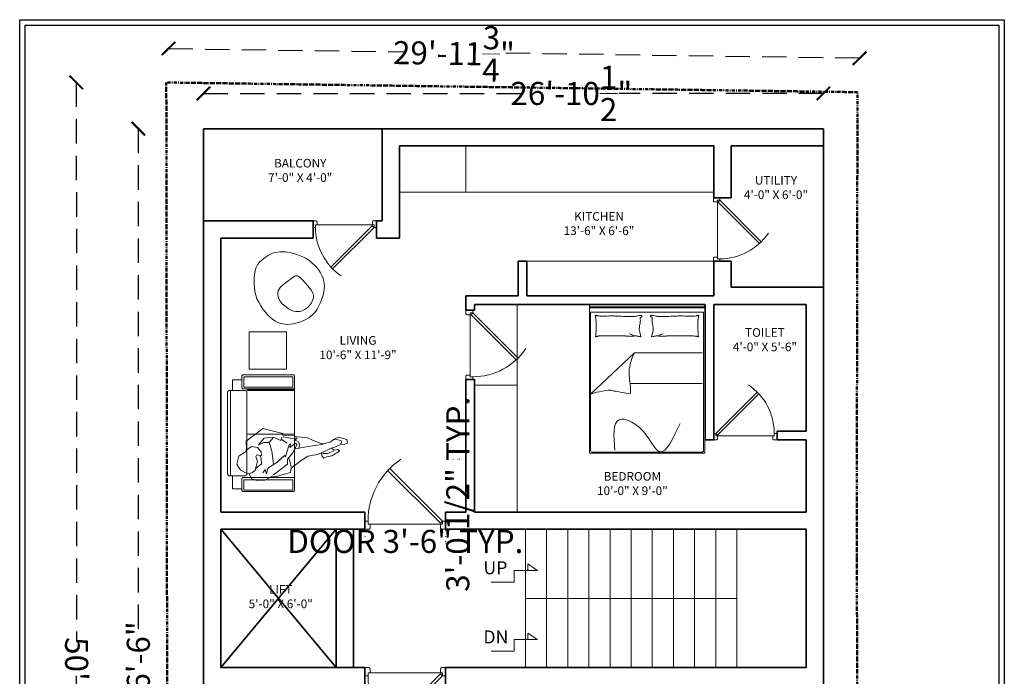
# Model space of a CAD drawing. Units: inches. Extents: x -16911 to -9621, y -48626 to -46270.
# Tile 3 of 20: x -16311 to -15799, y -46672 to -46330. Entities that reach past the tile are written whole.
import ezdxf

# ---------------------------------------------------------------- set-up
doc = ezdxf.new("R2010")
doc.units = ezdxf.units.IN
for name, pattern in [('DASHDOT', [1, 0.5, -0.25, 0, -0.25]), ('DASHED', [19.05, 12.7, -6.35]), ('DOT2', [3.175, 0, -3.175])]:
    doc.linetypes.add(name, pattern=pattern)
for name, color, linetype, lineweight in [('A-ANNO-DIMS', 2, 'Continuous', 13), ('A-ANNO-SYMB', 3, 'Continuous', 13), ('A-ANNO-TEXT', 7, 'Continuous', 18), ('A-ANNO-TTLB', 7, 'Continuous', 25), ('A-AREA-IDEN', 3, 'Continuous', 18), ('A-DOOR', 4, 'Continuous', 18), ('A-FLOR-STRS', 3, 'Continuous', 18), ('A-FURN', 8, 'Continuous', 13), ('A-WALL', 7, 'Continuous', 35), ('C-PROP', 6, 'DASHDOT', 50), ('DOOR', 143, 'Continuous', 9), ('furniture', 35, 'Continuous', 15), ('Man', 8, 'Continuous', 5), ('STAIRCASE', 137, 'Continuous', 5)]:
    doc.layers.add(name, color=color, linetype=linetype, lineweight=lineweight)
doc.styles.get("Standard").update_dxf_attribs({"font": 'swissel.ttf'})
doc.styles.add('style9', font='swisscl.ttf', dxfattribs={"height": 12})
doc.dimstyles.new('Dim9', dxfattribs={"dimtxt": 10, "dimasz": 0.199219, "dimexe": 1, "dimexo": 0.5, "dimgap": 1, "dimtad": 0, "dimdec": 1, "dimzin": 0, "dimdsep": 46, "dimlunit": 4, "dimtxsty": 'style9', "dimblk": 'ARCHTICK', "dimcen": 0.09, "dimclrd": 256, "dimclrt": 256, "dimadec": 0, "dimazin": 0, "dimtfac": 1, "dimtdec": 1, "dimtix": 1, "dimtofl": 0, "dimtmove": 1, "dimatfit": 3, "dimfxl": 9, "dimtolj": 1, "dimtzin": 0, "dimlwd": -1, "dimarcsym": 0})

# ---------------------------------------------------------------- blocks, each defined once
blk = doc.blocks.new('hjuyuiuyk')
at = {"layer": 'furniture'}
for p, q in [((-19327.49, -39738.98), (-19327.49, -39737.31)), ((-19327.49, -39737.31), (-19267.49, -39737.31, 0)), ((-19327.49, -39746.54), (-19327.49, -39737.31)), ((-19267.49, -39738.5), (-19327.49, -39738.5, 0)), ((-19327.49, -39738.5, 0), (-19327.49, -39814.72, 0)), ((-19327.49, -39738.5), (-19327.49, -39814.72)), ((-19267.49, -39738.5, 0), (-19327.49, -39738.5)), ((-19267.49, -39738.98, 0), (-19327.49, -39738.98)), ((-19267.49, -39737.31, 0), (-19267.49, -39738.98, 0)), ((-19267.49, -39746.54, 0), (-19267.49, -39737.31, 0)), ((-19267.49, -39814.72), (-19267.49, -39738.5)), ((-19267.49, -39814.72, 0), (-19267.49, -39738.5, 0)), ((-19268.1, -39741.33), (-19326.9, -39741.33)), ((-19326.9, -39741.33), (-19326.9, -39813.21)), ((-19268.1, -39813.21), (-19268.1, -39741.33)), ((-19300.88, -39753.22, 0), (-19301.49, -39750.81, 0)), ((-19300.67, -39754.09, 0), (-19300.88, -39753.22, 0)), ((-19295.19, -39754.09, 0), (-19294.97, -39753.22, 0)), ((-19294.97, -39753.22, 0), (-19294.37, -39750.81, 0)), ((-19304.07, -39762.52), (-19326.9, -39783.91)), ((-19304.07, -39762.52), (-19268.82, -39762.52)), ((-19268.82, -39778.34), (-19306.29, -39778.34)), ((-19326.9, -39813.21), (-19326.9, -39783.91)), ((-19327.49, -39814.72, 0), (-19267.49, -39814.72)), ((-19327.49, -39814.72), (-19267.49, -39814.72, 0)), ((-19269.1, -39814.21), (-19325.9, -39814.21)), ((-19325.9, -39814.21), (-19269.1, -39814.21))]:
    blk.add_line(p, q, dxfattribs=at)
for centre, radius, start, end in [((-19324.36, -39743.07, 0), 0.0997, 111.7883, 160.436), ((-19324.39, -39743.06, 0), 0.0676, 160.436, 281.8931), ((-19324.12, -39743.66, 0), 0.732, 94.3025, 111.7883), ((-19324.35, -39743.25, 0), 0.125, 21.9904, 101.8931), ((-19323.34, -39743.89, 0), 0.956, 158.579, 188.1335), ((-19317.18, -39743.01, 0), 7.17, 188.1335, 192.1095), ((-19324.65, -39743.37, 0), 0.455, 338.579, 21.9904), ((-19329.85, -39745.73, 0), 5.78, 7.6809, 12.1095), ((-19324.11, -39743.77, 0), 0.842, 59.3487, 94.3025), ((-19322.88, -39741.69, 0), 1.57, 239.3487, 264.7408), ((-19319.6, -39692.5, 0), 50.87, 266.1399, 268.6002), ((-19319.84, -39713.09, 0), 30.28, 268.0921, 271.2808), ((-19320.24, -39695.07, 0), 48.31, 271.2808, 273.4034), ((-19316.15, -39763.89, 0), 20.63, 90.1553, 93.4034), ((-19316.09, -39783.15, 0), 39.89, 86.9902, 90.1553), ((-19305.86, -39588.51, 0), 155.02, 266.9902, 268.5957), ((-19305.42, -39570.46, 0), 173.07, 268.5957, 270), ((-19305.42, -39718.38, 0), 25.15, 270, 273.6841), ((-19304.03, -39739.9, 0), 3.58, 273.6841, 287.1951), ((-19300.46, -39751.46, 0), 8.51, 98.4372, 107.1951), ((-19301.02, -39747.69, 0), 4.7, 90, 98.4372), ((-19301.12, -39743.14, 0), 0.997, 274.4002, 333.4195), ((-19315.3, -39745.68, 0), 14.34, 360, 6.2324), ((-19301.02, -39745.63, 0), 2.64, 78.7276, 90), ((-19300.58, -39743.42, 0), 0.383, 333.4195, 78.7276), ((-19295.28, -39743.42, 0), 0.383, 101.2724, 206.5805), ((-19294.73, -39743.14, 0), 0.997, 206.5805, 265.5998), ((-19294.84, -39745.63, 0), 2.64, 90, 101.2724), ((-19280.55, -39745.68, 0), 14.34, 173.7676, 180), ((-19294.84, -39747.69, 0), 4.7, 81.5628, 90), ((-19295.39, -39751.46, 0), 8.51, 72.8049, 81.5628), ((-19291.82, -39739.9, 0), 3.58, 252.8049, 266.3159), ((-19290.43, -39718.38, 0), 25.15, 266.3159, 270), ((-19290.43, -39570.46, 0), 173.07, 270, 271.4043), ((-19289.99, -39588.51, 0), 155.02, 271.4043, 273.0098), ((-19279.76, -39783.15, 0), 39.89, 89.8447, 93.0098), ((-19279.7, -39763.89, 0), 20.63, 86.5966, 89.8447), ((-19275.61, -39695.07, 0), 48.31, 266.5966, 268.7192), ((-19276.02, -39713.09, 0), 30.28, 268.7192, 271.9079), ((-19276.73, -39645.13, 0), 98.25, 271.0069, 272.7772), ((-19272.12, -39741.69, 0), 1.57, 275.2592, 300.6513), ((-19270.89, -39743.77, 0), 0.842, 85.6975, 120.6513), ((-19265.15, -39745.73, 0), 5.78, 167.8905, 172.3191), ((-19270.88, -39743.66, 0), 0.732, 68.2117, 85.6975), ((-19270.35, -39743.37, 0), 0.455, 158.0096, 201.421), ((-19277.82, -39743.01, 0), 7.17, 347.8905, 351.8665), ((-19270.65, -39743.25, 0), 0.125, 78.1069, 158.0096), ((-19271.66, -39743.89, 0), 0.956, 351.8665, 21.421), ((-19270.61, -39743.06, 0), 0.0676, 258.1069, 19.564), ((-19270.64, -39743.07, 0), 0.0997, 19.564, 68.2117), ((-19350.51, -39748.51, 0), 26.62, 3.3687, 7.6809), ((-19720.99, -39728.47, 0), 397.61, 356.4951, 356.945), ((-19363.7, -39747.54, 0), 39.81, 356.945, 358.3669), ((-19343.69, -39748.11, 0), 19.79, 358.3669, 3.3687), ((-19282.35, -39751.13, 0), 19.21, 171.9949, 177.3351), ((-19292.22, -39749.75, 0), 9.25, 167.8016, 171.9949), ((-19326.4, -39742.36, 0), 25.72, 347.8016, 350.3156), ((-19306.91, -39745.68, 0), 5.95, 350.3156, 360), ((-19288.94, -39745.68, 0), 5.95, 180, 189.6844), ((-19269.45, -39742.36, 0), 25.72, 189.6844, 192.1984), ((-19303.63, -39749.75, 0), 9.25, 8.0051, 12.1984), ((-19313.5, -39751.13, 0), 19.21, 2.6649, 8.0051), ((-19251.31, -39748.11, 0), 19.79, 176.6313, 181.6331), ((-19231.3, -39747.54, 0), 39.81, 181.6331, 183.055), ((-19244.49, -39748.51, 0), 26.62, 172.3191, 176.6313), ((-18874.01, -39728.47, 0), 397.61, 183.055, 183.5049), ((-19323.69, -39753.93, 0), 0.564, 170.0016, 196.6978), ((-19333.47, -39752.21, 0), 9.37, 350.0016, 356.4951), ((-19324.19, -39754.08, 0), 0.0385, 196.6978, 277.1204), ((-19324.51, -39751.59, 0), 2.55, 277.1204, 286.2212), ((-19324.42, -39751.9, 0), 2.23, 286.2212, 297.4439), ((-19322.81, -39754.99, 0), 1.25, 102.448, 117.4439), ((-19322.32, -39757.22, 0), 3.54, 93.574, 102.448), ((-19318.44, -39837.61, 0), 84.03, 90.9755, 92.7955), ((-19315.55, -39952.16, 0), 198.61, 89.4461, 91.2473), ((-19314.9, -39885.06, 0), 131.51, 87.2326, 89.4461), ((-19310.57, -39795.48, 0), 41.81, 85.4012, 87.2326), ((-19304.32, -39717.78, 0), 36.14, 265.4012, 267.3712), ((-19297.32, -39733.09, 0), 21.54, 244.6889, 246.5156), ((-19305.66, -39747.05, 0), 6.83, 267.3712, 281.4827), ((-19297.32, -39733.09, 0), 21.54, 246.5156, 248.3423), ((-19297.32, -39733.09, 0), 21.54, 248.3423, 250.572), ((-19297.32, -39733.09, 0), 21.54, 250.572, 252.8018), ((-19303.46, -39757.91, 0), 4.25, 83.5659, 101.4827), ((-19303.37, -39757.16, 0), 3.49, 72.6136, 83.5659), ((-19300.33, -39747.43, 0), 6.7, 252.6136, 260.5159), ((-19299.57, -39750.33, 0), 1.97, 177.3351, 194.0452), ((-19300.13, -39746.25, 0), 7.9, 260.5159, 265.9171), ((-19300.69, -39754.1, 0), 0.0267, 265.9171, 14.0449), ((-19295.16, -39754.1, 0), 0.0267, 165.9551, 274.0829), ((-19295.72, -39746.25, 0), 7.9, 274.0829, 279.4841), ((-19295.52, -39747.43, 0), 6.7, 279.4841, 287.3864), ((-19296.28, -39750.33, 0), 1.97, 345.9548, 2.6649), ((-19292.48, -39757.16, 0), 3.49, 96.4341, 107.3864), ((-19292.39, -39757.91, 0), 4.25, 78.5173, 96.4341), ((-19298.54, -39733.09, 0), 21.54, 287.1982, 289.428), ((-19290.19, -39747.05, 0), 6.83, 258.5173, 272.6288), ((-19298.54, -39733.09, 0), 21.54, 289.428, 291.6577), ((-19298.54, -39733.09, 0), 21.54, 291.6577, 293.4844), ((-19298.54, -39733.09, 0), 21.54, 293.4844, 295.3111), ((-19291.53, -39717.78, 0), 36.14, 272.6288, 274.5988), ((-19285.28, -39795.48, 0), 41.81, 92.7674, 94.5988), ((-19280.95, -39885.06, 0), 131.51, 90.5539, 92.7674), ((-19280.3, -39952.16, 0), 198.61, 88.7527, 90.5539), ((-19277.1, -39805.01, 0), 51.42, 86.426, 88.7527), ((-19274.68, -39799.75, 0), 46.07, 86.5575, 89.0171), ((-19272.19, -39754.99, 0), 1.25, 62.5561, 77.552), ((-19270.58, -39751.9, 0), 2.23, 242.5561, 253.7788), ((-19270.49, -39751.59, 0), 2.55, 253.7788, 262.8796), ((-19261.53, -39752.21, 0), 9.37, 183.5049, 189.9984), ((-19270.81, -39754.08, 0), 0.0385, 262.8796, 343.3022), ((-19271.31, -39753.93, 0), 0.564, 343.3022, 9.9984), ((-19279.47, -39774.89), 27.53, 153.3084, 168.7423), ((-19287.94, -39773.2), 18.89, 168.7423, 187.3994), ((-19242.78, -39767.34), 64.43, 187.3994, 189.2719), ((-19333.07, -39782.08), 27.05, 6.3817, 9.2719), ((-19321.79, -39780.82), 15.7, 359.2313, 6.3817), ((-19306.77, -39846.83), 66.07, 105.9352, 107.7364), ((-19318.41, -39806.06), 23.67, 102.9255, 105.9352), ((-19287.64, -39956.87), 177.57, 99.7243, 101.7196), ((-19317.24, -39783.9), 2.09, 82.2696, 100.7276), ((-19317.9, -39788.76), 6.99, 76.8096, 82.2696), ((-19295.64, -39693.77), 90.57, 256.8096, 258.3259), ((-19295.11, -39691.23), 93.17, 258.3259, 260.505), ((-19288.03, -39648.9), 136.08, 260.505, 262.308), ((-19336.71, -39780.62), 30.63, 354.1141, 359.2313), ((-19325.9, -39813.21), 1, 180, 270), ((-19269.1, -39813.21), 1, 270, 0)]:
    blk.add_arc(centre, radius, start, end, dxfattribs=at)
blk.add_open_spline([(-19280.24, -39799.21), (-19283.87, -39806.94), (-19290.73, -39821.55), (-19298.08, -39801.09), (-19315.85, -39793.47), (-19314.86, -39805.92), (-19314.29, -39813.13)], degree=3, knots=[0, 0, 0, 0, 18.167809, 34.338432, 45.972904, 61.997799, 61.997799, 61.997799, 61.997799], dxfattribs=at)
blk = doc.blocks.new('Bipman02')
blk.add_lwpolyline([(0.5871, -0.067), (0.6175, -0.0496), (0.6523, -0.0539), (0.6697, -0.0376), (0.5958, 0.0069), (0.5437, 0.0156), (0.5164, 0.0297), (0.4959, 0.0069), (0.4915, -0.0235), (0.4524, -0.0061), (0.3568, 0.0113), (0.2917, 0.0548), (0.1917, 0.1287), (0.1874, 0.1722), (0.031, 0.2156), (0.0049, 0.2069), (-0.0689, 0.2461), (-0.1471, 0.2504), (-0.1949, 0.233), (-0.2253, 0.1808), (-0.2384, 0.1852), (-0.3079, 0.1504), (-0.3426, 0.0895), (-0.3253, 0.0113), (-0.2558, -0.0365), (-0.2471, -0.0583), (-0.2514, -0.1365), (-0.0863, -0.2626), (0.1092, -0.2148), (0.1092, -0.193), (0.2265, -0.1974), (0.2308, -0.1844), (0.3525, -0.1713), (0.409, -0.1452), (0.4872, -0.1148), (0.5089, -0.1104), (0.5828, -0.1322), (0.6088, -0.1496), (0.6295, -0.1636), (0.661, -0.1757), (0.7435, -0.1539), (0.7478, -0.1191), (0.7143, -0.1051), (0.674, -0.1017), (0.6392, -0.0844)], close=True)
for points in [[(-0.2558, -0.0452), (-0.1993, -0.0844), (-0.1385, -0.0757), (-0.1037, -0.0322), (-0.0994, 0.0069), (-0.1471, -0.0018), (-0.1558, 0.0156), (-0.1385, 0.0591), (-0.1515, 0.1113), (-0.1645, 0.1504), (-0.1906, 0.1722), (-0.2167, 0.1808)], [(-0.1558, 0.133), (-0.0994, 0.0852), (-0.1037, 0.033), (-0.1124, 0.0069)], [(-0.0863, 0.1765), (-0.0646, 0.1417), (-0.0516, 0.1895), (-0.0385, 0.1287), (0.0527, 0.0722), (0.1266, 0.0026), (0.1353, 0.0156), (0.1744, -0.1061), (0.1874, -0.1104), (0.1787, -0.0757), (0.2352, -0.1191), (0.2482, -0.1061), (0.2091, -0.0235), (0.157, 0.0417), (0.157, 0.0895), (0.018, 0.1939)], [(0.1917, 0.1156), (0.1744, 0.0374)], [(0.018, 0.0895), (0.0006, -0.0409), (-0.0255, -0.1235), (-0.0776, -0.1235), (-0.1298, -0.1017), (-0.0733, -0.167), (0.0136, -0.1757), (0.0918, -0.1452), (0.1005, -0.1757)], [(0.2699, -0.0757), (0.2743, -0.0974), (0.2699, -0.1278), (0.2439, -0.1409), (0.2222, -0.1452), (0.2482, -0.1626), (0.2482, -0.1713), (0.2004, -0.1626), (0.1135, -0.18)], [(0.2308, -0.0626), (0.3612, -0.0844), (0.5089, -0.1095)], [(0.4915, -0.0235), (0.5871, -0.067)], [(0.5045, -0.0148), (0.5523, -0.0148), (0.6132, -0.0409)], [(-0.0255, -0.1235), (0.0136, -0.1713)], [(0.0962, -0.1539), (0.1526, -0.1191)], [(0.6783, -0.1104), (0.6914, -0.1278), (0.687, -0.1409), (0.6566, -0.1496), (0.6088, -0.1539)]]:
    blk.add_lwpolyline(points)
blk = doc.blocks.new('erertety')
at = {"layer": 'furniture', "ltscale": 0.2}
for p, q in [((-17662.13, -45230.66), (-17662.13, -45176.69)), ((-17693.83, -45223.2), (-17693.83, -45184.43)), ((-17685.49, -45183.68), (-17693.08, -45183.68)), ((-17684.74, -45223.2), (-17684.74, -45184.43)), ((-17684.74, -45203.31), (-17662.13, -45203.31)), ((-17685.49, -45223.95), (-17693.08, -45223.95)), ((-17691.58, -45223.95), (-17691.58, -45229.1)), ((-17684.74, -45223.99), (-17662.13, -45223.99)), ((-17684.74, -45224.55), (-17662.13, -45224.55)), ((-17684.74, -45224.55), (-17662.13, -45224.55)), ((-17691.58, -45229.1), (-17687.09, -45229.1))]:
    blk.add_line(p, q, dxfattribs=at)
for points in [[(-17662.13, -45182.17), (-17662.13, -45176.97, 0.414214), (-17662.87, -45176.22), (-17686.34, -45176.22, 0.414214), (-17687.09, -45176.97), (-17687.09, -45182.17, 0.414214), (-17686.34, -45182.91), (-17662.87, -45182.91, 0.414214)], [(-17662.13, -45225.47), (-17662.13, -45230.66, -0.414214), (-17662.87, -45231.41), (-17686.34, -45231.41, -0.414214), (-17687.09, -45230.66), (-17687.09, -45225.47, -0.414214), (-17686.34, -45224.72), (-17662.87, -45224.72, -0.414214)]]:
    blk.add_lwpolyline(points, format="xyb", close=True, dxfattribs=at)
for points in [[(-17663.01, -45181.75), (-17663.01, -45176.82), (-17686.21, -45176.82), (-17686.21, -45181.75)], [(-17692.4, -45183.68), (-17692.4, -45223.95), (-17692.4, -45223.95), (-17692.4, -45183.68)], [(-17663.01, -45225.6), (-17663.01, -45230.53), (-17686.21, -45230.53), (-17686.21, -45225.6)]]:
    blk.add_lwpolyline(points, close=True, dxfattribs=at)
blk.add_lwpolyline([(-17687.09, -45177.54), (-17691.58, -45177.54), (-17691.58, -45183.68)], dxfattribs=at)
for centre, start, end in [((-17693.08, -45184.43), 90, 180), ((-17685.49, -45184.43), 0, 90), ((-17693.08, -45223.2), 180, 270), ((-17685.49, -45223.2), 270, 0)]:
    blk.add_arc(centre, 0.748, start, end, dxfattribs=at)
at = {"layer": 'furniture', "ltscale": 0.2, "xscale": 47.90818138957024, "yscale": 47.90818138957024, "zscale": 47.90818138957024}
blk.add_blockref('Bipman02', (-17673, -45193.44, 0), dxfattribs=at)
blk = doc.blocks.new('rthrty')
at = {"layer": 'furniture'}
blk.add_open_spline([(-17650.3, -45154.53), (-17651.97, -45142.9), (-17645.3, -45136.31), (-17637.11, -45132.37), (-17620.71, -45137.17), (-17612.47, -45149.45), (-17615.73, -45159.71), (-17619.67, -45168.02), (-17632.28, -45172.65), (-17641.84, -45170.43), (-17649.5, -45159.42), (-17650.3, -45154.53)], degree=3, dxfattribs=at)
at = {"layer": 'Man'}
blk.add_open_spline([(-17632.99, -45149.02), (-17629.89, -45146.6), (-17628, -45145.12), (-17623.29, -45151.15), (-17618.06, -45156.77), (-17623.15, -45164.08), (-17628.28, -45165.32), (-17631.61, -45164.6), (-17638.01, -45159.61), (-17638.81, -45154.69), (-17636.9, -45151.81), (-17632.99, -45149.02), (-17632.99, -45149.02)], degree=3, dxfattribs=at)
blk = doc.blocks.new('A$C1C9D3E54')
at = {"layer": 'DOOR'}
blk.add_line((18676.53, 5780.72), (18710.53, 5780.72), dxfattribs=at)
blk.add_lwpolyline([(18685.01, 5806.62), (18710.47, 5781.16), (18711.53, 5782.22), (18686.07, 5807.68), (18685.01, 5806.62)], dxfattribs=at)
blk.add_lwpolyline([(18674.03, 5778.22), (18676.03, 5778.22), (18674.03, 5778.22), (18674.03, 5782.22), (18675.53, 5782.22), (18675.53, 5780.72), (18676.53, 5780.72), (18676.53, 5778.72), (18676.41, 5778.72), (18676.41, 5778.6, -0.414214), (18676.16, 5778.35), (18676.03, 5778.35), (18676.03, 5778.22)], format="xyb", dxfattribs=at)
blk.add_lwpolyline([(18713.03, 5782.22), (18711.53, 5782.22), (18711.53, 5780.72), (18710.53, 5780.72), (18710.53, 5778.72), (18710.66, 5778.72), (18710.66, 5778.6, 0.414214), (18710.91, 5778.35), (18711.03, 5778.35), (18711.03, 5778.22), (18713.03, 5778.22), (18711.03, 5778.22), (18713.03, 5778.22), (18713.03, 5782.22)], format="xyb", close=True, dxfattribs=at)
blk.add_arc((18711.53, 5782.22), 36, 124.0336, 180, dxfattribs=at)
blk = doc.blocks.new('_ArchTick')
at = {"color": 0, "linetype": 'ByBlock', "const_width": 0.15}
blk.add_lwpolyline([(-0.5, -0.5), (0.5, 0.5)], dxfattribs=at)
blk = doc.blocks.new('*D57')
at = {"layer": 'A-ANNO-DIMS', "color": 0, "linetype": 'DOT2', "lineweight": -2, "transparency": 16777216}
for p, q in [((-16234.02, -46345.34), (-16234, -46344.15)), ((-15874.35, -46350.39), (-15874.34, -46349.2))]:
    blk.add_line(p, q, dxfattribs=at)
at = {"layer": 'A-ANNO-DIMS', "color": 0, "linetype": 'DASHED', "lineweight": 25, "transparency": 16777216}
for p, q in [((-16234.01, -46345.15), (-16110.27, -46346.89)), ((-15874.35, -46350.2), (-16060.69, -46347.59))]:
    blk.add_line(p, q, dxfattribs=at)
at = {"layer": 'Defpoints', "color": 0, "transparency": 16777216}
for p in [(-15874.35, -46350.2), (-16234.21, -46359.07), (-15874.55, -46364.11)]:
    blk.add_point(p, dxfattribs=at)
at = {"layer": 'A-ANNO-DIMS', "color": 0, "lineweight": 25, "transparency": 16777216, "xscale": 7, "yscale": 7, "zscale": 7}
for p, rotation in [((-16234.01, -46345.15), 179.1963905603631), ((-15874.35, -46350.2), 359.196390560363)]:
    blk.add_blockref('_ArchTick', p, dxfattribs=dict(at, rotation=rotation))
at = {"layer": 'A-ANNO-DIMS', "color": 0, "transparency": 16777216, "insert": (-16085.49, -46347.68), "char_height": 12, "attachment_point": 5, "rotation": 359.1964, "style": 'style9'}
blk.add_mtext('\\A1;29\'-11{\\H1x;\\S3/4;}"', dxfattribs=at)
blk = doc.blocks.new('*D58')
at = {"layer": 'A-ANNO-DIMS', "color": 0, "linetype": 'DOT2', "lineweight": -2, "transparency": 16777216}
for p, q in [((-16281.81, -46362.82), (-16283, -46362.82)), ((-16281.44, -46962.82), (-16282.63, -46962.82))]:
    blk.add_line(p, q, dxfattribs=at)
at = {"layer": 'A-ANNO-DIMS', "color": 0, "linetype": 'DASHED', "lineweight": 25, "transparency": 16777216}
for p, q in [((-16282, -46362.82), (-16281.82, -46653.98)), ((-16281.63, -46962.82), (-16281.81, -46671.67))]:
    blk.add_line(p, q, dxfattribs=at)
at = {"layer": 'Defpoints', "color": 0, "transparency": 16777216}
for p in [(-16282, -46362.82), (-16263.18, -46362.81), (-16262.82, -46962.81)]:
    blk.add_point(p, dxfattribs=at)
at = {"layer": 'A-ANNO-DIMS', "color": 0, "lineweight": 25, "transparency": 16777216, "xscale": 7, "yscale": 7, "zscale": 7}
for p, rotation in [((-16282, -46362.82), 90.0346840750536), ((-16281.63, -46962.82), 270.0346840750536)]:
    blk.add_blockref('_ArchTick', p, dxfattribs=dict(at, rotation=rotation))
at = {"layer": 'A-ANNO-DIMS', "color": 0, "transparency": 16777216, "insert": (-16281.81, -46662.82), "char_height": 12, "attachment_point": 5, "rotation": 270.0347, "style": 'style9'}
blk.add_mtext("\\A1;50'", dxfattribs=at)
blk = doc.blocks.new('*D59')
at = {"layer": 'A-ANNO-DIMS', "color": 0, "linetype": 'DOT2', "lineweight": -2, "transparency": 16777216}
for p, q in [((-16215.78, -46368.33), (-16215.78, -46369.52)), ((-15893.23, -46368.33), (-15893.23, -46369.52))]:
    blk.add_line(p, q, dxfattribs=at)
at = {"layer": 'A-ANNO-DIMS', "color": 0, "linetype": 'DASHED', "lineweight": 25, "transparency": 16777216}
for p, q in [((-16215.78, -46368.52), (-16049, -46368.52)), ((-15893.23, -46368.52), (-15999.73, -46368.52))]:
    blk.add_line(p, q, dxfattribs=at)
at = {"layer": 'Defpoints', "color": 0, "transparency": 16777216}
for p in [(-16215.78, -46345.28), (-15893.23, -46345.28), (-15893.23, -46368.52)]:
    blk.add_point(p, dxfattribs=at)
at = {"layer": 'A-ANNO-DIMS', "color": 0, "lineweight": 25, "transparency": 16777216, "xscale": 7, "yscale": 7, "zscale": 7, "rotation": 180}
blk.add_blockref('_ArchTick', (-16215.78, -46368.52), dxfattribs=at)
at = {"layer": 'A-ANNO-DIMS', "color": 0, "lineweight": 25, "transparency": 16777216, "xscale": 7, "yscale": 7, "zscale": 7}
blk.add_blockref('_ArchTick', (-15893.23, -46368.52), dxfattribs=at)
at = {"layer": 'A-ANNO-DIMS', "color": 0, "transparency": 16777216, "insert": (-16024.37, -46368.52), "char_height": 12, "attachment_point": 5, "style": 'style9'}
blk.add_mtext('\\A1;26\'-10{\\H1x;\\S1/2;}"', dxfattribs=at)
blk = doc.blocks.new('*D60')
at = {"layer": 'A-ANNO-DIMS', "color": 0, "linetype": 'DOT2', "lineweight": -2, "transparency": 16777216}
for p, q in [((-16249.52, -46386.86), (-16250.71, -46386.86)), ((-16249.52, -46944.81), (-16250.71, -46944.81))]:
    blk.add_line(p, q, dxfattribs=at)
at = {"layer": 'A-ANNO-DIMS', "color": 0, "linetype": 'DASHED', "lineweight": 25, "transparency": 16777216}
for p, q in [((-16249.71, -46386.86), (-16249.71, -46648.2)), ((-16249.71, -46944.81), (-16249.71, -46683.47))]:
    blk.add_line(p, q, dxfattribs=at)
at = {"layer": 'Defpoints', "color": 0, "transparency": 16777216}
for p in [(-16215.78, -46386.86), (-16249.71, -46944.81), (-16215.78, -46944.81)]:
    blk.add_point(p, dxfattribs=at)
at = {"layer": 'A-ANNO-DIMS', "color": 0, "lineweight": 25, "transparency": 16777216, "xscale": 7, "yscale": 7, "zscale": 7}
for p, rotation in [((-16249.71, -46386.86), 90), ((-16249.71, -46944.81), 270)]:
    blk.add_blockref('_ArchTick', p, dxfattribs=dict(at, rotation=rotation))
at = {"layer": 'A-ANNO-DIMS', "color": 0, "transparency": 16777216, "insert": (-16249.71, -46665.83), "char_height": 12, "attachment_point": 5, "rotation": 90, "style": 'style9'}
blk.add_mtext('\\A1;46\'-6"', dxfattribs=at)
blk = doc.blocks.new('THYHYTJ')
at = {"layer": 'STAIRCASE', "ltscale": 10}
for p, q in [((-7981.18, -46346.18), (-7984.62, -46351.1)), ((-7981.18, -46358.18), (-7981.18, -46346.18)), ((-7984.62, -46351.1), (-7981.18, -46351.1)), ((-7975.18, -46358.18), (-7981.18, -46358.18)), ((-7975.18, -46370.18), (-7975.18, -46358.18))]:
    blk.add_line(p, q, dxfattribs=at)
blk = doc.blocks.new('TITLE-BLOCK-A3')
for p, q in [((-16311.44, -47065.27), (-16311.44, -46330.13)), ((-16311.44, -46330.13), (-15799.07, -46330.13)), ((-16308.66, -47062.49), (-16308.66, -46332.91)), ((-16308.66, -46332.91), (-15801.86, -46332.91)), ((-15801.86, -46332.91), (-15801.86, -47062.49)), ((-15799.07, -46330.13), (-15799.07, -47065.27))]:
    blk.add_line(p, q)
blk = doc.blocks.new('*D69')
at = {"layer": 'A-ANNO-DIMS', "color": 0, "linetype": 'DOT2', "lineweight": -2, "transparency": 16777216}
for p, q in [((-16131.78, -46595.86), (-16131.78, -46602.66)), ((-16089.78, -46595.86), (-16089.78, -46602.66))]:
    blk.add_line(p, q, dxfattribs=at)
at = {"layer": 'A-ANNO-DIMS', "linetype": 'DASHED', "transparency": 16777216}
for p, q in [((-16131.78, -46601.66), (-16131.98, -46601.66)), ((-16089.78, -46601.66), (-16089.58, -46601.66))]:
    blk.add_line(p, q, dxfattribs=at)
at = {"layer": 'Defpoints', "color": 0, "transparency": 16777216}
for p in [(-16131.78, -46595.36), (-16089.78, -46595.36), (-16089.78, -46601.66)]:
    blk.add_point(p, dxfattribs=at)
at = {"layer": 'A-ANNO-DIMS', "transparency": 16777216, "xscale": 0.19921875, "yscale": 0.19921875, "zscale": 0.19921875}
blk.add_blockref('_ArchTick', (-16131.78, -46601.66), dxfattribs=at)
at = {"layer": 'A-ANNO-DIMS', "transparency": 16777216, "xscale": 0.19921875, "yscale": 0.19921875, "zscale": 0.19921875, "rotation": 180}
blk.add_blockref('_ArchTick', (-16089.78, -46601.66), dxfattribs=at)
at = {"layer": 'A-ANNO-DIMS', "transparency": 16777216, "insert": (-16110.78, -46601.66), "char_height": 12, "attachment_point": 5, "style": 'style9'}
blk.add_mtext('\\A1;DOOR 3\'-6" TYP.', dxfattribs=at)
blk = doc.blocks.new('*D70')
at = {"layer": 'A-ANNO-DIMS', "color": 0, "linetype": 'DOT2', "lineweight": -2, "transparency": 16777216}
for p, q in [((-16089.28, -46558.92), (-16082.48, -46558.92)), ((-16089.28, -46595.36), (-16082.48, -46595.36))]:
    blk.add_line(p, q, dxfattribs=at)
at = {"layer": 'A-ANNO-DIMS', "linetype": 'DASHED', "transparency": 16777216}
for p, q in [((-16083.48, -46558.92), (-16083.48, -46558.72)), ((-16083.48, -46595.36), (-16083.48, -46595.55))]:
    blk.add_line(p, q, dxfattribs=at)
at = {"layer": 'Defpoints', "color": 0, "transparency": 16777216}
for p in [(-16089.78, -46558.92), (-16083.48, -46558.92), (-16089.78, -46595.36)]:
    blk.add_point(p, dxfattribs=at)
at = {"layer": 'A-ANNO-DIMS', "transparency": 16777216, "xscale": 0.19921875, "yscale": 0.19921875, "zscale": 0.19921875}
for p, rotation in [((-16083.48, -46558.92), 270), ((-16083.48, -46595.36), 90)]:
    blk.add_blockref('_ArchTick', p, dxfattribs=dict(at, rotation=rotation))
at = {"layer": 'A-ANNO-DIMS', "transparency": 16777216, "insert": (-16083.48, -46577.14), "char_height": 12, "attachment_point": 5, "rotation": 90, "style": 'style9'}
blk.add_mtext('\\A1;3\'-0 1/2" TYP.', dxfattribs=at)

msp = doc.modelspace()

# ---------------------------------------------------------------- linework, layer by layer
at = {"layer": 'A-FLOR-STRS', "ltscale": 10}
for p, q in [((-16048.233, -46595.355), (-16048.233, -46667.355)), ((-16037.233, -46595.355), (-16037.233, -46667.355)), ((-16026.233, -46595.355), (-16026.233, -46667.355)), ((-16015.233, -46595.355), (-16015.233, -46667.355)), ((-16004.233, -46595.355), (-16004.233, -46667.355)), ((-15993.233, -46595.355), (-15993.233, -46667.355)), ((-15982.233, -46595.355), (-15982.233, -46667.355)), ((-15971.233, -46595.355), (-15971.233, -46667.355)), ((-15960.233, -46595.355), (-15960.233, -46667.355)), ((-15949.233, -46595.355), (-15949.233, -46667.355)), ((-15938.233, -46595.355), (-15938.233, -46667.355)), ((-15938.233, -46631.355), (-16048.233, -46631.355))]:
    msp.add_line(p, q, dxfattribs=at)
at = {"layer": 'A-FURN', "ltscale": 0.2}
for p, q in [((-16079.283, -46419.855), (-16079.283, -46395.855)), ((-15950.233, -46419.855), (-16113.783, -46419.855)), ((-15950.233, -46455.855), (-16047.533, -46455.855)), ((-16074.783, -46520.355), (-16052.533, -46520.355)), ((-16052.533, -46520.355), (-16052.533, -46586.355))]:
    msp.add_line(p, q, dxfattribs=at)
at = {"layer": 'A-FURN', "ltscale": 0.5}
msp.add_line((-16052.533, -46520.355), (-16052.533, -46478.355), dxfattribs=at)
at = {"layer": 'A-FURN'}
msp.add_lwpolyline([(-16172.662, -46511.978), (-16192.022, -46511.978), (-16192.022, -46492.618), (-16172.662, -46492.618)], close=True, dxfattribs=at)
at = {"layer": 'A-WALL'}
for p, q in [((-16215.783, -46434.855), (-16215.783, -46386.855)), ((-16122.783, -46386.855), (-16215.783, -46386.855)), ((-16122.783, -46434.855), (-16122.783, -46386.855)), ((-15893.233, -46386.855), (-16122.783, -46386.855)), ((-15893.233, -46386.855), (-15893.233, -46395.855)), ((-16113.783, -46443.855), (-16113.783, -46395.855)), ((-15950.233, -46395.855), (-16113.783, -46395.855)), ((-15950.233, -46395.855), (-15950.233, -46422.855)), ((-15893.233, -46395.855), (-15941.233, -46395.855)), ((-15941.233, -46395.855), (-15941.233, -46422.855)), ((-15893.233, -46395.855), (-15893.233, -46469.355)), ((-15950.233, -46422.855), (-15941.233, -46422.855)), ((-16215.783, -46896.809), (-16215.783, -46434.855)), ((-16158.783, -46434.855), (-16215.783, -46434.855)), ((-16158.783, -46434.855), (-16158.783, -46443.855)), ((-16122.783, -46434.855), (-16125.783, -46434.855)), ((-16125.783, -46434.855), (-16125.783, -46443.855)), ((-16206.783, -46586.355), (-16206.783, -46443.855)), ((-16158.783, -46443.855), (-16206.783, -46443.855)), ((-16113.783, -46443.855), (-16125.783, -46443.855)), ((-16052.033, -46473.855), (-16052.033, -46455.855)), ((-16047.533, -46455.855), (-16052.033, -46455.855)), ((-16047.533, -46473.855), (-16047.533, -46455.855)), ((-15950.233, -46455.855), (-15950.233, -46473.855)), ((-15950.233, -46455.855), (-15941.233, -46455.855)), ((-15941.233, -46455.855), (-15941.233, -46469.355)), ((-15893.233, -46469.355), (-15941.233, -46469.355)), ((-15893.233, -46469.355), (-15893.233, -46676.355)), ((-16079.283, -46481.355), (-16079.283, -46473.855)), ((-16052.033, -46473.855), (-16079.283, -46473.855)), ((-15950.233, -46473.855), (-16047.533, -46473.855)), ((-16079.283, -46481.355), (-16074.783, -46481.355)), ((-16074.783, -46481.355), (-16074.783, -46478.355)), ((-15954.733, -46478.355), (-16074.783, -46478.355)), ((-15954.733, -46478.355), (-15954.733, -46548.855)), ((-15902.233, -46478.355), (-15950.233, -46478.355)), ((-15950.233, -46478.355), (-15950.233, -46548.855)), ((-15902.233, -46478.355), (-15902.233, -46544.355)), ((-16079.283, -46586.355), (-16079.283, -46517.355)), ((-16079.283, -46517.355), (-16074.783, -46517.355)), ((-16074.783, -46586.355), (-16074.783, -46517.355)), ((-15950.233, -46548.855), (-15954.733, -46548.855)), ((-15902.233, -46544.355), (-15917.233, -46544.355)), ((-15917.233, -46544.355), (-15917.233, -46548.855)), ((-15902.233, -46548.855), (-15917.233, -46548.855)), ((-15902.233, -46548.855), (-15902.233, -46586.355)), ((-16131.783, -46586.355), (-16206.783, -46586.355)), ((-16131.783, -46595.355), (-16131.783, -46586.355)), ((-16079.283, -46586.355), (-16089.783, -46586.355)), ((-16089.783, -46595.355), (-16089.783, -46586.355)), ((-15902.233, -46586.355), (-16074.783, -46586.355)), ((-16206.783, -46667.355), (-16206.783, -46595.355)), ((-16131.783, -46595.355), (-16206.783, -46595.355)), ((-16206.783, -46595.355), (-16146.783, -46667.355)), ((-16206.783, -46667.355), (-16146.783, -46595.355)), ((-16146.783, -46667.355), (-16146.783, -46595.355)), ((-16137.783, -46667.355), (-16137.783, -46595.355)), ((-15902.233, -46595.355), (-16089.783, -46595.355)), ((-15902.233, -46595.355), (-15902.233, -46667.355)), ((-16131.783, -46667.355), (-16206.783, -46667.355)), ((-16131.783, -46676.355), (-16131.783, -46667.355)), ((-15902.233, -46667.355), (-16089.783, -46667.355)), ((-16089.783, -46676.355), (-16089.783, -46667.355))]:
    msp.add_line(p, q, dxfattribs=at)
at = {"layer": 'C-PROP'}
msp.add_lwpolyline([(-16234.783, -46962.809), (-15874.601, -46969.035), (-15874.04, -46940.446), (-15874.703, -46855.606), (-15875.869, -46609.511), (-15875.483, -46367.855), (-16235.146, -46362.811), (-16234.608, -46762.955)], close=True, dxfattribs=at)

# ---------------------------------------------------------------- block references
at = {"layer": 'A-ANNO-SYMB', "rotation": 270.0000000000144}
for p in [(30304.121, -54597.957), (30304.121, -54633.957)]:
    msp.add_blockref('THYHYTJ', p, dxfattribs=at)
at = {"layer": 'A-ANNO-TTLB'}
msp.add_blockref('TITLE-BLOCK-A3', (0, 0), dxfattribs=at)
at = {"layer": 'A-DOOR'}
for p, xscale, yscale, zscale, rotation in [((-20839.75, -62256.958), -0.8461538461538624, 0.8461538461538624, 0.8461538461538624, 270), ((-31959.886, -41545.589), -0.8461538461538624, 0.8461538461538624, 0.8461538461538624, 180), ((-21413.028, -63754.922), -0.9230769230769229, 0.9230769230769229, 0.9230769230769229, 270), ((-36242.277, -40444.653), -1.076923076922859, 1.076923076922859, 1.076923076922859, 180)]:
    msp.add_blockref('A$C1C9D3E54', p, dxfattribs=dict(at, xscale=xscale, yscale=yscale, zscale=zscale, rotation=rotation))
for p, xscale, yscale, zscale in [((-116.38, -51438.122), -0.8461538461538624, 0.8461538461538624, 0.8461538461538624), ((-36242.277, -52818.058), 1.076923076922859, 1.076923076922859, 1.076923076922859)]:
    msp.add_blockref('A$C1C9D3E54', p, dxfattribs=dict(at, xscale=xscale, yscale=yscale, zscale=zscale))
at = {"layer": 'A-FURN'}
for name, p in [('rthrty', (1461.229, -1317.075)), ('hjuyuiuyk', (3312.503, -6741.043, 0))]:
    msp.add_blockref(name, p, dxfattribs=at)
at = {"layer": 'A-FURN', "xscale": -1.1, "yscale": 1.1, "zscale": 1.1, "rotation": 180}
msp.add_blockref('erertety', (3259.977, -96269.509, 0), dxfattribs=at)

# ---------------------------------------------------------------- texts
at = {"layer": 'A-ANNO-TEXT'}
for s, p in [('UP', (-16070.133, -46618.742)), ('DN', (-16070.133, -46654.742))]:
    msp.add_text(s, height=6.75, dxfattribs=at).set_placement(p)
at = {"layer": 'A-AREA-IDEN', "ltscale": 10, "char_height": 4.5, "width": 42.823, "attachment_point": 1, "style": 'style9'}
for s, insert in [('\\A1;\\pxqc;{\\fCentury Gothic|b0|i0|c0|p34;BALCONY\\P7\'-0" X 4\'-0"}', (-16186.876, -46402.553)), ('\\A1;\\pxqc;{\\fCentury Gothic|b0|i0|c0|p34;UTILITY\\P4\'-0" X 6\'-0"}', (-15939.305, -46411.463)), ('\\A1;\\pxqc;{\\fCentury Gothic|b0|i0|c0|p34;KITCHEN\\P13\'-6" X 6\'-6"}', (-16031.398, -46430.204)), ('\\A1;\\pxqc;{\\fCentury Gothic|b0|i0|c0|p34;TOILET\\P4\'-0" X 5\'-6"}', (-15945.056, -46490.664)), ('\\A1;\\pxqc;{\\fCentury Gothic|b0|i0|c0|p34;LIVING\\P10\'-6" X 11\'-9"}', (-16156.795, -46494.801)), ('\\A1;\\pxqc;{\\fCentury Gothic|b0|i0|c0|p34;BEDROOM\\P10\'-0" X 9\'-0"}', (-16014.034, -46565.526)), ('\\A1;\\pxqc;{\\fCentury Gothic|b0|i0|c0|p34;LIFT\\P5\'-0" X 6\'-0"}', (-16197.007, -46624.39))]:
    msp.add_mtext(s, dxfattribs=dict(at, insert=insert))

# ---------------------------------------------------------------- dimensions: what is measured, and where the dimension line sits
at = {"layer": 'A-ANNO-DIMS'}
dim = msp.add_linear_dim(base=(-15874.352, -46350.199), p1=(-16234.21, -46359.069), p2=(-15874.547, -46364.114), angle=359.19639, dimstyle='Dim9', override={"dimtxt": 12, "dimasz": 7, "dimdec": 2, "dimclrd": 0, "dimclre": 0, "dimclrt": 0, "dimtdec": 2, "dimfxl": 0.1875, "dimfxlon": 1, "dimlwd": 25, "dimarcsym": 2}, dxfattribs=at)
dim.commit()
dim.dimension.update_dxf_attribs({"geometry": '*D57', "text_midpoint": (-16085.488, -46347.677), "dimtype": 161})
dim = msp.add_linear_dim(base=(-15893.233, -46368.516), p1=(-16215.783, -46345.28), p2=(-15893.233, -46345.28), dimstyle='Dim9', override={"dimtxt": 12, "dimasz": 7, "dimdec": 2, "dimclrd": 0, "dimclre": 0, "dimclrt": 0, "dimtdec": 2, "dimfxl": 0.1875, "dimfxlon": 1, "dimlwd": 25, "dimarcsym": 2}, dxfattribs=at)
dim.commit()
dim.dimension.update_dxf_attribs({"geometry": '*D59', "text_midpoint": (-16024.367, -46368.516), "dimtype": 160})
dim = msp.add_aligned_dim(p1=(-16262.815, -46962.809), p2=(-16263.178, -46362.811), distance=18.817, dimstyle='Dim9', override={"dimtxt": 12, "dimasz": 7, "dimdec": 2, "dimclrd": 0, "dimclre": 0, "dimclrt": 0, "dimtdec": 2, "dimfxl": 0.1875, "dimfxlon": 1, "dimlwd": 25, "dimarcsym": 2}, dxfattribs=at)
dim.commit()
dim.dimension.update_dxf_attribs({"geometry": '*D58', "text_midpoint": (-16281.814, -46662.821)})
dim = msp.add_linear_dim(base=(-16249.711, -46944.809), p1=(-16215.783, -46386.855), p2=(-16215.783, -46944.809), angle=90, dimstyle='Dim9', override={"dimtxt": 12, "dimasz": 7, "dimdec": 2, "dimclrd": 0, "dimclre": 0, "dimclrt": 0, "dimtdec": 2, "dimfxl": 0.1875, "dimfxlon": 1, "dimlwd": 25, "dimarcsym": 2}, dxfattribs=at)
dim.commit()
dim.dimension.update_dxf_attribs({"geometry": '*D60', "text_midpoint": (-16249.711, -46665.832)})
dim = msp.add_linear_dim(base=(-16083.483, -46558.924), p1=(-16089.783, -46595.355), p2=(-16089.783, -46558.924), angle=90, text='<> TYP.', dimstyle='Dim9', override={"dimdec": 1, "dimrnd": 0, "dimzin": 1, "dimlunit": 4, "dimfrac": 2}, dxfattribs=at)
dim.commit()
dim.dimension.update_dxf_attribs({"geometry": '*D70', "text_midpoint": (-16083.483, -46577.14)})
dim = msp.add_linear_dim(base=(-16089.783, -46601.655), p1=(-16131.783, -46595.355), p2=(-16089.783, -46595.355), text='DOOR <> TYP.', dimstyle='Dim9', override={"dimdec": 1, "dimrnd": 0, "dimzin": 1, "dimlunit": 4, "dimfrac": 2}, dxfattribs=at)
dim.commit()
dim.dimension.update_dxf_attribs({"geometry": '*D69', "text_midpoint": (-16110.783, -46601.655)})

doc.saveas('drawing.dxf')
